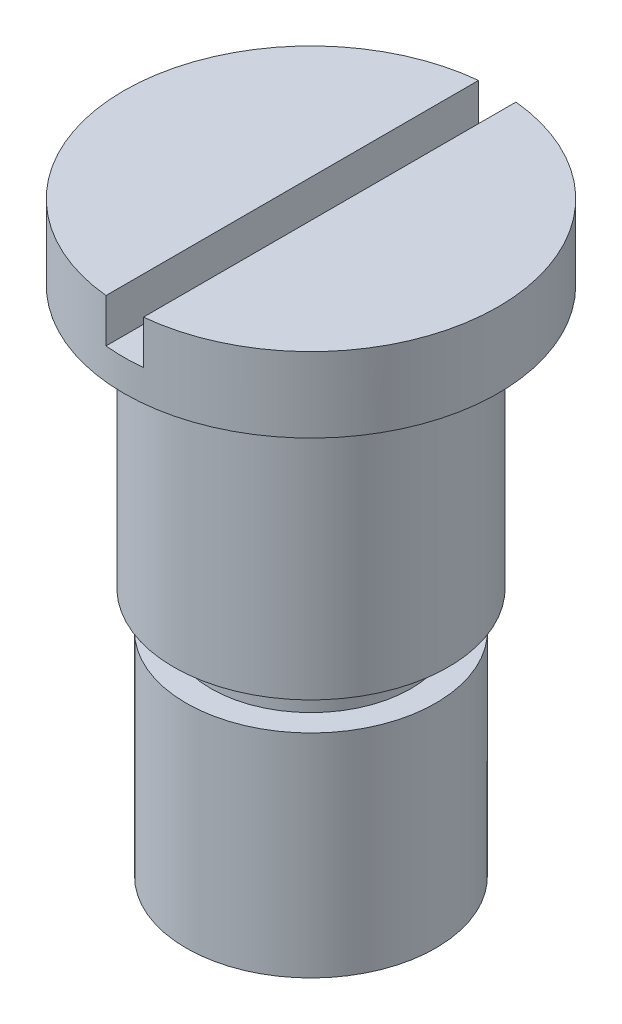
ISO-10303-21;
HEADER;
FILE_DESCRIPTION(('STEP AP214'),'2;1');
FILE_NAME('part.step','',(''),(''),'','','');
FILE_SCHEMA(('AUTOMOTIVE_DESIGN { 1 0 10303 214 1 1 1 1 }'));
ENDSEC;
DATA;
#1=APPLICATION_CONTEXT('core data for automotive mechanical design processes');
#2=APPLICATION_PROTOCOL_DEFINITION('international standard','automotive_design',2000,#1);
#3=PRODUCT_CONTEXT('',#1,'mechanical');
#4=PRODUCT('Part','Part','',(#3));
#5=PRODUCT_RELATED_PRODUCT_CATEGORY('part','',(#4));
#6=PRODUCT_DEFINITION_FORMATION('','',#4);
#7=PRODUCT_DEFINITION_CONTEXT('part definition',#1,'design');
#8=PRODUCT_DEFINITION('design','',#6,#7);
#9=PRODUCT_DEFINITION_SHAPE('','',#8);
#10=(LENGTH_UNIT() NAMED_UNIT(*) SI_UNIT(.MILLI.,.METRE.));
#11=(NAMED_UNIT(*) PLANE_ANGLE_UNIT() SI_UNIT($,.RADIAN.));
#12=(NAMED_UNIT(*) SI_UNIT($,.STERADIAN.) SOLID_ANGLE_UNIT());
#13=UNCERTAINTY_MEASURE_WITH_UNIT(LENGTH_MEASURE(1.E-05),#10,'distance_accuracy_value','');
#14=(GEOMETRIC_REPRESENTATION_CONTEXT(3) GLOBAL_UNCERTAINTY_ASSIGNED_CONTEXT((#13)) GLOBAL_UNIT_ASSIGNED_CONTEXT((#10,
#11,#12)) REPRESENTATION_CONTEXT('',''));
#15=CARTESIAN_POINT('',(0.,0.,0.));
#16=DIRECTION('',(0.,0.,1.));
#17=DIRECTION('',(1.,0.,0.));
#18=AXIS2_PLACEMENT_3D('',#15,#16,#17);
#19=CARTESIAN_POINT('',(0.,47.,0.));
#20=DIRECTION('',(0.,1.,0.));
#21=DIRECTION('',(0.,0.,1.));
#22=AXIS2_PLACEMENT_3D('',#19,#20,#21);
#23=PLANE('',#22);
#24=DIRECTION('',(0.,0.,1.));
#25=VECTOR('',#24,1.);
#26=CARTESIAN_POINT('',(-1.5,47.,0.));
#27=LINE('',#26,#25);
#28=CARTESIAN_POINT('',(-1.5,47.,-14.9248115565993));
#29=VERTEX_POINT('',#28);
#30=CARTESIAN_POINT('',(-1.5,47.,14.9248115565993));
#31=VERTEX_POINT('',#30);
#32=EDGE_CURVE('E88',#29,#31,#27,.T.);
#33=ORIENTED_EDGE('',*,*,#32,.F.);
#34=CARTESIAN_POINT('',(0.,47.,0.));
#35=DIRECTION('',(0.,1.,0.));
#36=DIRECTION('',(0.,0.,1.));
#37=AXIS2_PLACEMENT_3D('',#34,#35,#36);
#38=CIRCLE('',#37,15.);
#39=EDGE_CURVE('E99',#29,#31,#38,.T.);
#40=ORIENTED_EDGE('',*,*,#39,.T.);
#41=EDGE_LOOP('',(#33,#40));
#42=FACE_BOUND('',#41,.T.);
#43=ADVANCED_FACE('F39',(#42),#23,.T.);
#44=CARTESIAN_POINT('',(0.,17.,0.));
#45=DIRECTION('',(0.,-1.,0.));
#46=DIRECTION('',(0.,0.,-1.));
#47=AXIS2_PLACEMENT_3D('',#44,#45,#46);
#48=CYLINDRICAL_SURFACE('',#47,10.);
#49=CARTESIAN_POINT('',(0.,17.,0.));
#50=DIRECTION('',(0.,1.,0.));
#51=DIRECTION('',(0.,0.,1.));
#52=AXIS2_PLACEMENT_3D('',#49,#50,#51);
#53=CIRCLE('',#52,10.);
#54=CARTESIAN_POINT('',(0.,17.,10.));
#55=VERTEX_POINT('',#54);
#56=EDGE_CURVE('E123',#55,#55,#53,.T.);
#57=ORIENTED_EDGE('',*,*,#56,.F.);
#58=EDGE_LOOP('',(#57));
#59=FACE_BOUND('',#58,.T.);
#60=CARTESIAN_POINT('',(0.,0.,0.));
#61=DIRECTION('',(0.,1.,0.));
#62=DIRECTION('',(0.,0.,1.));
#63=AXIS2_PLACEMENT_3D('',#60,#61,#62);
#64=CIRCLE('',#63,10.);
#65=CARTESIAN_POINT('',(0.,0.,10.));
#66=VERTEX_POINT('',#65);
#67=EDGE_CURVE('E116',#66,#66,#64,.T.);
#68=ORIENTED_EDGE('',*,*,#67,.T.);
#69=EDGE_LOOP('',(#68));
#70=FACE_BOUND('',#69,.T.);
#71=ADVANCED_FACE('F41',(#59,#70),#48,.T.);
#72=CARTESIAN_POINT('',(0.,17.,0.));
#73=DIRECTION('',(0.,1.,0.));
#74=DIRECTION('',(0.,0.,1.));
#75=AXIS2_PLACEMENT_3D('',#72,#73,#74);
#76=PLANE('',#75);
#77=CARTESIAN_POINT('',(0.,17.,0.));
#78=DIRECTION('',(0.,1.,0.));
#79=DIRECTION('',(0.,0.,1.));
#80=AXIS2_PLACEMENT_3D('',#77,#78,#79);
#81=CIRCLE('',#80,8.);
#82=CARTESIAN_POINT('',(0.,17.,8.));
#83=VERTEX_POINT('',#82);
#84=EDGE_CURVE('E87',#83,#83,#81,.T.);
#85=ORIENTED_EDGE('',*,*,#84,.F.);
#86=EDGE_LOOP('',(#85));
#87=FACE_BOUND('',#86,.T.);
#88=ORIENTED_EDGE('',*,*,#56,.T.);
#89=EDGE_LOOP('',(#88));
#90=FACE_BOUND('',#89,.T.);
#91=ADVANCED_FACE('F142',(#87,#90),#76,.T.);
#92=CARTESIAN_POINT('',(0.,0.,0.));
#93=DIRECTION('',(0.,1.,0.));
#94=DIRECTION('',(0.,0.,1.));
#95=AXIS2_PLACEMENT_3D('',#92,#93,#94);
#96=PLANE('',#95);
#97=ORIENTED_EDGE('',*,*,#67,.F.);
#98=EDGE_LOOP('',(#97));
#99=FACE_BOUND('',#98,.T.);
#100=ADVANCED_FACE('F170',(#99),#96,.F.);
#101=CARTESIAN_POINT('',(0.,20.,0.));
#102=DIRECTION('',(0.,-1.,0.));
#103=DIRECTION('',(0.,0.,-1.));
#104=AXIS2_PLACEMENT_3D('',#101,#102,#103);
#105=CYLINDRICAL_SURFACE('',#104,8.);
#106=CARTESIAN_POINT('',(0.,20.,0.));
#107=DIRECTION('',(0.,1.,0.));
#108=DIRECTION('',(0.,0.,1.));
#109=AXIS2_PLACEMENT_3D('',#106,#107,#108);
#110=CIRCLE('',#109,8.);
#111=CARTESIAN_POINT('',(0.,20.,8.));
#112=VERTEX_POINT('',#111);
#113=EDGE_CURVE('E111',#112,#112,#110,.T.);
#114=ORIENTED_EDGE('',*,*,#113,.F.);
#115=EDGE_LOOP('',(#114));
#116=FACE_BOUND('',#115,.T.);
#117=ORIENTED_EDGE('',*,*,#84,.T.);
#118=EDGE_LOOP('',(#117));
#119=FACE_BOUND('',#118,.T.);
#120=ADVANCED_FACE('F162',(#116,#119),#105,.T.);
#121=CARTESIAN_POINT('',(0.,41.,0.));
#122=DIRECTION('',(0.,-1.,0.));
#123=DIRECTION('',(0.,0.,-1.));
#124=AXIS2_PLACEMENT_3D('',#121,#122,#123);
#125=CYLINDRICAL_SURFACE('',#124,11.);
#126=CARTESIAN_POINT('',(0.,41.,0.));
#127=DIRECTION('',(0.,1.,0.));
#128=DIRECTION('',(0.,0.,1.));
#129=AXIS2_PLACEMENT_3D('',#126,#127,#128);
#130=CIRCLE('',#129,11.);
#131=CARTESIAN_POINT('',(0.,41.,-11.));
#132=VERTEX_POINT('',#131);
#133=EDGE_CURVE('E103',#132,#132,#130,.T.);
#134=CARTESIAN_POINT('',(0.,20.,0.));
#135=DIRECTION('',(0.,1.,0.));
#136=DIRECTION('',(0.,0.,1.));
#137=AXIS2_PLACEMENT_3D('',#134,#135,#136);
#138=CIRCLE('',#137,11.);
#139=CARTESIAN_POINT('',(0.,20.,-11.));
#140=VERTEX_POINT('',#139);
#141=EDGE_CURVE('E97',#140,#140,#138,.T.);
#142=CARTESIAN_POINT('',(0.,41.,-11.));
#143=CARTESIAN_POINT('',(0.,40.78125,-11.));
#144=CARTESIAN_POINT('',(0.,40.5625,-11.));
#145=CARTESIAN_POINT('',(0.,40.125,-11.));
#146=CARTESIAN_POINT('',(0.,39.90625,-11.));
#147=CARTESIAN_POINT('',(0.,39.46875,-11.));
#148=CARTESIAN_POINT('',(0.,39.25,-11.));
#149=CARTESIAN_POINT('',(0.,38.8125,-11.));
#150=CARTESIAN_POINT('',(0.,38.59375,-11.));
#151=CARTESIAN_POINT('',(0.,38.15625,-11.));
#152=CARTESIAN_POINT('',(0.,37.9375,-11.));
#153=CARTESIAN_POINT('',(0.,37.5,-11.));
#154=CARTESIAN_POINT('',(0.,37.28125,-11.));
#155=CARTESIAN_POINT('',(0.,36.84375,-11.));
#156=CARTESIAN_POINT('',(0.,36.625,-11.));
#157=CARTESIAN_POINT('',(0.,36.1875,-11.));
#158=CARTESIAN_POINT('',(0.,35.96875,-11.));
#159=CARTESIAN_POINT('',(0.,35.53125,-11.));
#160=CARTESIAN_POINT('',(0.,35.3125,-11.));
#161=CARTESIAN_POINT('',(0.,34.875,-11.));
#162=CARTESIAN_POINT('',(0.,34.65625,-11.));
#163=CARTESIAN_POINT('',(0.,34.21875,-11.));
#164=CARTESIAN_POINT('',(0.,34.,-11.));
#165=CARTESIAN_POINT('',(0.,33.5625,-11.));
#166=CARTESIAN_POINT('',(0.,33.34375,-11.));
#167=CARTESIAN_POINT('',(0.,32.90625,-11.));
#168=CARTESIAN_POINT('',(0.,32.6875,-11.));
#169=CARTESIAN_POINT('',(0.,32.25,-11.));
#170=CARTESIAN_POINT('',(0.,32.03125,-11.));
#171=CARTESIAN_POINT('',(0.,31.59375,-11.));
#172=CARTESIAN_POINT('',(0.,31.375,-11.));
#173=CARTESIAN_POINT('',(0.,30.9375,-11.));
#174=CARTESIAN_POINT('',(0.,30.71875,-11.));
#175=CARTESIAN_POINT('',(0.,30.28125,-11.));
#176=CARTESIAN_POINT('',(0.,30.0625,-11.));
#177=CARTESIAN_POINT('',(0.,29.625,-11.));
#178=CARTESIAN_POINT('',(0.,29.40625,-11.));
#179=CARTESIAN_POINT('',(0.,28.96875,-11.));
#180=CARTESIAN_POINT('',(0.,28.75,-11.));
#181=CARTESIAN_POINT('',(0.,28.3125,-11.));
#182=CARTESIAN_POINT('',(0.,28.09375,-11.));
#183=CARTESIAN_POINT('',(0.,27.65625,-11.));
#184=CARTESIAN_POINT('',(0.,27.4375,-11.));
#185=CARTESIAN_POINT('',(0.,27.,-11.));
#186=CARTESIAN_POINT('',(0.,26.78125,-11.));
#187=CARTESIAN_POINT('',(0.,26.34375,-11.));
#188=CARTESIAN_POINT('',(0.,26.125,-11.));
#189=CARTESIAN_POINT('',(0.,25.6875,-11.));
#190=CARTESIAN_POINT('',(0.,25.46875,-11.));
#191=CARTESIAN_POINT('',(0.,25.03125,-11.));
#192=CARTESIAN_POINT('',(0.,24.8125,-11.));
#193=CARTESIAN_POINT('',(0.,24.375,-11.));
#194=CARTESIAN_POINT('',(0.,24.15625,-11.));
#195=CARTESIAN_POINT('',(0.,23.71875,-11.));
#196=CARTESIAN_POINT('',(0.,23.5,-11.));
#197=CARTESIAN_POINT('',(0.,23.0625,-11.));
#198=CARTESIAN_POINT('',(0.,22.84375,-11.));
#199=CARTESIAN_POINT('',(0.,22.40625,-11.));
#200=CARTESIAN_POINT('',(0.,22.1875,-11.));
#201=CARTESIAN_POINT('',(0.,21.75,-11.));
#202=CARTESIAN_POINT('',(0.,21.53125,-11.));
#203=CARTESIAN_POINT('',(0.,21.09375,-11.));
#204=CARTESIAN_POINT('',(0.,20.875,-11.));
#205=CARTESIAN_POINT('',(0.,20.4375,-11.));
#206=CARTESIAN_POINT('',(0.,20.21875,-11.));
#207=CARTESIAN_POINT('',(0.,20.,-11.));
#208=B_SPLINE_CURVE_WITH_KNOTS('',3,(#142,#143,#144,#145,#146,#147,#148,#149,#150,#151,#152,
#153,#154,#155,#156,#157,#158,#159,#160,#161,#162,#163,#164,#165,#166,#167,#168,#169,#170,#171,
#172,#173,#174,#175,#176,#177,#178,#179,#180,#181,#182,#183,#184,#185,#186,#187,#188,#189,#190,
#191,#192,#193,#194,#195,#196,#197,#198,#199,#200,#201,#202,#203,#204,#205,#206,#207),
.UNSPECIFIED.,.F.,.F.,(4,2,2,2,2,2,2,2,2,2,2,2,2,2,2,2,2,2,2,2,2,2,2,2,2,2,2,2,2,2,2,2,4),(0.,
0.656250000000004,1.3125,1.96875000000001,2.625,3.28125000000001,3.9375,4.59375,5.25,5.90625,
6.56250000000001,7.21875,7.875,8.53125,9.1875,9.84375,10.5,11.15625,11.8125,12.46875,13.125,
13.78125,14.4375,15.09375,15.75,16.40625,17.0625,17.71875,18.375,19.03125,19.6875,20.34375,21.),.UNSPECIFIED.);
#209=EDGE_CURVE('BSEAM160',#132,#140,#208,.T.);
#210=ORIENTED_EDGE('',*,*,#133,.F.);
#211=ORIENTED_EDGE('',*,*,#141,.T.);
#212=ORIENTED_EDGE('',*,*,#209,.T.);
#213=ORIENTED_EDGE('',*,*,#209,.F.);
#214=EDGE_LOOP('',(#210,#212,#211,#213));
#215=FACE_BOUND('',#214,.T.);
#216=ADVANCED_FACE('F160',(#215),#125,.T.);
#217=CARTESIAN_POINT('',(0.,20.,0.));
#218=DIRECTION('',(0.,1.,0.));
#219=DIRECTION('',(0.,0.,1.));
#220=AXIS2_PLACEMENT_3D('',#217,#218,#219);
#221=PLANE('',#220);
#222=ORIENTED_EDGE('',*,*,#113,.T.);
#223=EDGE_LOOP('',(#222));
#224=FACE_BOUND('',#223,.T.);
#225=ORIENTED_EDGE('',*,*,#141,.F.);
#226=EDGE_LOOP('',(#225));
#227=FACE_BOUND('',#226,.T.);
#228=ADVANCED_FACE('F155',(#224,#227),#221,.F.);
#229=CARTESIAN_POINT('',(0.,47.,0.));
#230=DIRECTION('',(0.,-1.,0.));
#231=DIRECTION('',(0.,0.,-1.));
#232=AXIS2_PLACEMENT_3D('',#229,#230,#231);
#233=CYLINDRICAL_SURFACE('',#232,15.);
#234=ORIENTED_EDGE('',*,*,#39,.F.);
#235=DIRECTION('',(0.,-1.,0.));
#236=VECTOR('',#235,1.);
#237=CARTESIAN_POINT('',(-1.5,47.,-14.9248115565993));
#238=LINE('',#237,#236);
#239=CARTESIAN_POINT('',(-1.5,43.5,-14.9248115565993));
#240=VERTEX_POINT('',#239);
#241=EDGE_CURVE('E108',#29,#240,#238,.T.);
#242=ORIENTED_EDGE('',*,*,#241,.T.);
#243=CARTESIAN_POINT('',(0.,43.5,0.));
#244=DIRECTION('',(0.,1.,0.));
#245=DIRECTION('',(0.,0.,1.));
#246=AXIS2_PLACEMENT_3D('',#243,#244,#245);
#247=CIRCLE('',#246,15.);
#248=CARTESIAN_POINT('',(1.5,43.5,-14.9248115565993));
#249=VERTEX_POINT('',#248);
#250=EDGE_CURVE('E11',#249,#240,#247,.T.);
#251=ORIENTED_EDGE('',*,*,#250,.F.);
#252=DIRECTION('',(0.,-1.,0.));
#253=VECTOR('',#252,1.);
#254=CARTESIAN_POINT('',(1.5,47.,-14.9248115565993));
#255=LINE('',#254,#253);
#256=CARTESIAN_POINT('',(1.5,47.,-14.9248115565993));
#257=VERTEX_POINT('',#256);
#258=EDGE_CURVE('E83',#249,#257,#255,.F.);
#259=ORIENTED_EDGE('',*,*,#258,.T.);
#260=CARTESIAN_POINT('',(1.5,47.,14.9248115565993));
#261=VERTEX_POINT('',#260);
#262=EDGE_CURVE('E94',#261,#257,#38,.T.);
#263=ORIENTED_EDGE('',*,*,#262,.F.);
#264=DIRECTION('',(0.,-1.,0.));
#265=VECTOR('',#264,1.);
#266=CARTESIAN_POINT('',(1.5,47.,14.9248115565993));
#267=LINE('',#266,#265);
#268=CARTESIAN_POINT('',(1.5,43.5,14.9248115565993));
#269=VERTEX_POINT('',#268);
#270=EDGE_CURVE('E53',#261,#269,#267,.T.);
#271=ORIENTED_EDGE('',*,*,#270,.T.);
#272=CARTESIAN_POINT('',(-1.5,43.5,14.9248115565993));
#273=VERTEX_POINT('',#272);
#274=EDGE_CURVE('E43',#273,#269,#247,.T.);
#275=ORIENTED_EDGE('',*,*,#274,.F.);
#276=DIRECTION('',(0.,-1.,0.));
#277=VECTOR('',#276,1.);
#278=CARTESIAN_POINT('',(-1.5,47.,14.9248115565993));
#279=LINE('',#278,#277);
#280=EDGE_CURVE('E65',#273,#31,#279,.F.);
#281=ORIENTED_EDGE('',*,*,#280,.T.);
#282=EDGE_LOOP('',(#234,#242,#251,#259,#263,#271,#275,#281));
#283=FACE_BOUND('',#282,.T.);
#284=CARTESIAN_POINT('',(0.,41.,0.));
#285=DIRECTION('',(0.,1.,0.));
#286=DIRECTION('',(0.,0.,1.));
#287=AXIS2_PLACEMENT_3D('',#284,#285,#286);
#288=CIRCLE('',#287,15.);
#289=CARTESIAN_POINT('',(0.,41.,15.));
#290=VERTEX_POINT('',#289);
#291=EDGE_CURVE('E106',#290,#290,#288,.T.);
#292=ORIENTED_EDGE('',*,*,#291,.T.);
#293=EDGE_LOOP('',(#292));
#294=FACE_BOUND('',#293,.T.);
#295=ADVANCED_FACE('F95',(#283,#294),#233,.T.);
#296=DIRECTION('',(0.,0.,-1.));
#297=VECTOR('',#296,1.);
#298=CARTESIAN_POINT('',(1.5,47.,0.));
#299=LINE('',#298,#297);
#300=EDGE_CURVE('E76',#261,#257,#299,.T.);
#301=ORIENTED_EDGE('',*,*,#300,.F.);
#302=ORIENTED_EDGE('',*,*,#262,.T.);
#303=EDGE_LOOP('',(#301,#302));
#304=FACE_BOUND('',#303,.T.);
#305=ADVANCED_FACE('F98',(#304),#23,.T.);
#306=CARTESIAN_POINT('',(0.,41.,0.));
#307=DIRECTION('',(0.,1.,0.));
#308=DIRECTION('',(0.,0.,1.));
#309=AXIS2_PLACEMENT_3D('',#306,#307,#308);
#310=PLANE('',#309);
#311=ORIENTED_EDGE('',*,*,#133,.T.);
#312=EDGE_LOOP('',(#311));
#313=FACE_BOUND('',#312,.T.);
#314=ORIENTED_EDGE('',*,*,#291,.F.);
#315=EDGE_LOOP('',(#314));
#316=FACE_BOUND('',#315,.T.);
#317=ADVANCED_FACE('F150',(#313,#316),#310,.F.);
#318=CARTESIAN_POINT('',(0.,43.5,0.));
#319=DIRECTION('',(0.,1.,0.));
#320=DIRECTION('',(0.,0.,1.));
#321=AXIS2_PLACEMENT_3D('',#318,#319,#320);
#322=PLANE('',#321);
#323=ORIENTED_EDGE('',*,*,#250,.T.);
#324=DIRECTION('',(0.,0.,1.));
#325=VECTOR('',#324,1.);
#326=CARTESIAN_POINT('',(-1.5,43.5,-16.1902823413104));
#327=LINE('',#326,#325);
#328=EDGE_CURVE('E129',#240,#273,#327,.T.);
#329=ORIENTED_EDGE('',*,*,#328,.T.);
#330=ORIENTED_EDGE('',*,*,#274,.T.);
#331=DIRECTION('',(0.,0.,-1.));
#332=VECTOR('',#331,1.);
#333=CARTESIAN_POINT('',(1.5,43.5,-16.1902823413104));
#334=LINE('',#333,#332);
#335=EDGE_CURVE('E96',#269,#249,#334,.T.);
#336=ORIENTED_EDGE('',*,*,#335,.T.);
#337=EDGE_LOOP('',(#323,#329,#330,#336));
#338=FACE_BOUND('',#337,.T.);
#339=ADVANCED_FACE('F126',(#338),#322,.T.);
#340=CARTESIAN_POINT('',(-1.5,43.5,-16.1902823413104));
#341=DIRECTION('',(-1.,0.,0.));
#342=DIRECTION('',(0.,0.,1.));
#343=AXIS2_PLACEMENT_3D('',#340,#341,#342);
#344=PLANE('',#343);
#345=ORIENTED_EDGE('',*,*,#32,.T.);
#346=ORIENTED_EDGE('',*,*,#280,.F.);
#347=ORIENTED_EDGE('',*,*,#328,.F.);
#348=ORIENTED_EDGE('',*,*,#241,.F.);
#349=EDGE_LOOP('',(#345,#346,#347,#348));
#350=FACE_BOUND('',#349,.T.);
#351=ADVANCED_FACE('F131',(#350),#344,.F.);
#352=CARTESIAN_POINT('',(1.5,43.5,-16.1902823413104));
#353=DIRECTION('',(1.,0.,0.));
#354=DIRECTION('',(0.,0.,-1.));
#355=AXIS2_PLACEMENT_3D('',#352,#353,#354);
#356=PLANE('',#355);
#357=ORIENTED_EDGE('',*,*,#300,.T.);
#358=ORIENTED_EDGE('',*,*,#258,.F.);
#359=ORIENTED_EDGE('',*,*,#335,.F.);
#360=ORIENTED_EDGE('',*,*,#270,.F.);
#361=EDGE_LOOP('',(#357,#358,#359,#360));
#362=FACE_BOUND('',#361,.T.);
#363=ADVANCED_FACE('F79',(#362),#356,.F.);
#364=CLOSED_SHELL('',(#43,#71,#91,#100,#120,#216,#228,#295,#305,#317,#339,#351,#363));
#365=MANIFOLD_SOLID_BREP('B2',#364);
#366=ADVANCED_BREP_SHAPE_REPRESENTATION('',(#18,#365),#14);
#367=SHAPE_DEFINITION_REPRESENTATION(#9,#366);
ENDSEC;
END-ISO-10303-21;
